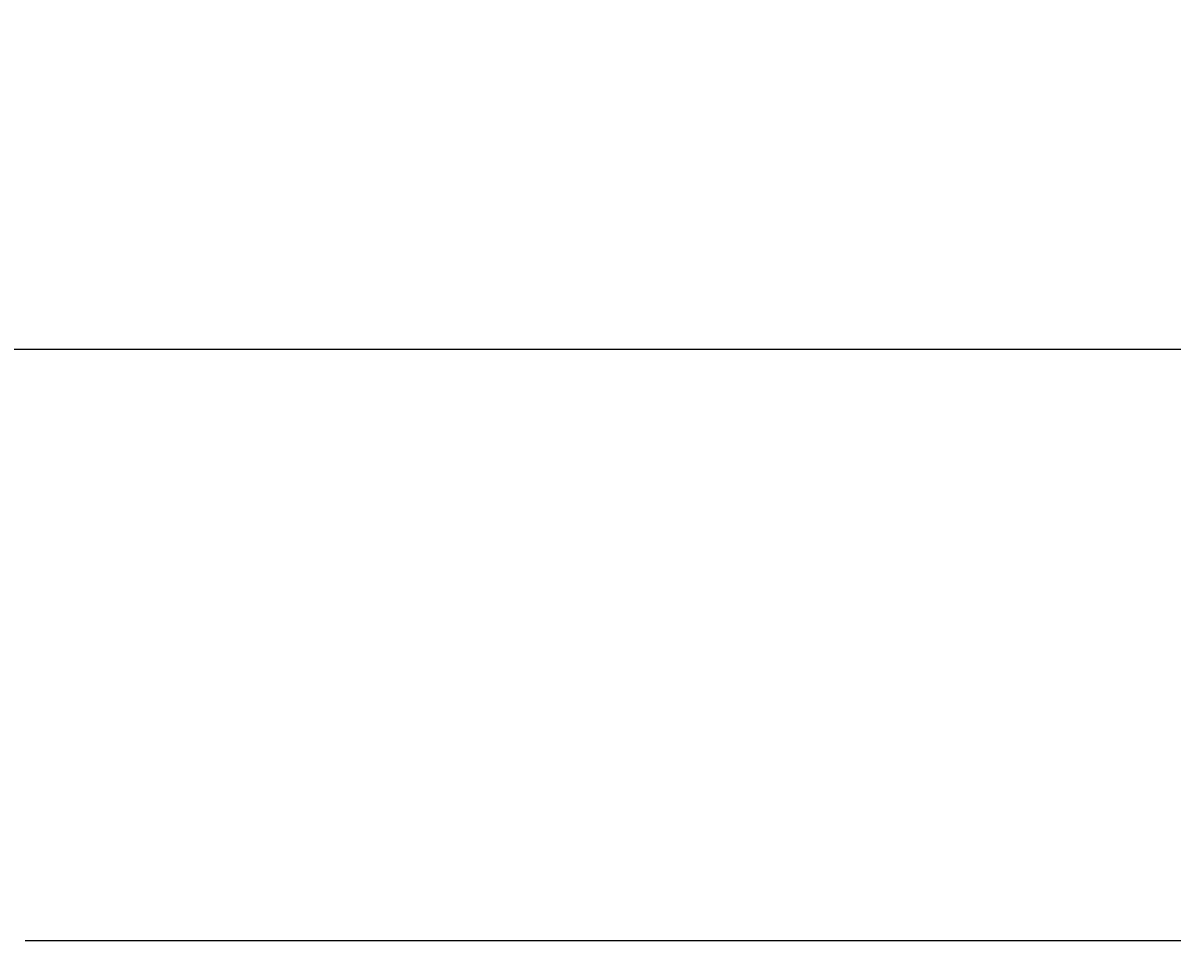
# Model space of a CAD drawing. Units: inches. Extents: x 1998 to 2588, y 1139 to 1977.
# Tile 11 of 134: x 2115 to 2147, y 1596 to 1622. Entities that reach past the tile are written whole.
import ezdxf

# ---------------------------------------------------------------- set-up
doc = ezdxf.new("R2010")
doc.units = ezdxf.units.IN
doc.layers.add('A-ANNO-DIMS', color=2, linetype='Continuous', lineweight=18)
doc.styles.get("Standard").update_dxf_attribs({"font": 'arial.ttf'})
doc.dimstyles.get("Standard").update_dxf_attribs({"dimtxt": 0.18, "dimasz": 0.18, "dimexe": 0.18, "dimexo": 0.0625, "dimgap": 0.09, "dimtad": 0, "dimtih": 1, "dimtoh": 1, "dimdec": 4, "dimzin": 0, "dimdsep": 46, "dimtxsty": 'Standard', "dimcen": 0.09, "dimadec": 0, "dimazin": 0, "dimtfac": 1, "dimtdec": 4, "dimtofl": 0, "dimtmove": 0, "dimatfit": 3, "dimfxl": 1, "dimtolj": 1, "dimtzin": 0, "dimarcsym": 0})

# ---------------------------------------------------------------- blocks, each defined once
blk = doc.blocks.new('*D30')
at = {"layer": 'A-ANNO-DIMS', "color": 0, "lineweight": -2, "transparency": 16777216}
for p, q in [((2407.91, 1636.732), (1997.843, 1636.732)), ((1998.023, 1636.552), (1998.023, 1615.913)), ((1998.023, 1594.912), (1998.023, 1615.552)), ((2407.91, 1594.732), (1997.843, 1594.732))]:
    blk.add_line(p, q, dxfattribs=at)
at = {"layer": 'A-ANNO-DIMS', "color": 0, "transparency": 16777216}
for points in [[(1997.993, 1636.552), (1998.053, 1636.552), (1998.023, 1636.732)], [(1997.993, 1594.912), (1998.053, 1594.912), (1998.023, 1594.732)]]:
    blk.add_solid(points, dxfattribs=at)
at = {"layer": 'Defpoints', "color": 0, "transparency": 16777216}
for p in [(1998.023, 1636.732), (2407.973, 1636.732), (2407.973, 1594.732)]:
    blk.add_point(p, dxfattribs=at)
at = {"layer": 'A-ANNO-DIMS', "color": 0, "transparency": 16777216, "insert": (1998.023, 1615.732), "char_height": 0.18, "attachment_point": 5}
blk.add_mtext('\\A1;42', dxfattribs=at)
blk = doc.blocks.new('*D35')
at = {"layer": 'A-ANNO-DIMS', "color": 0, "lineweight": -2, "transparency": 16777216}
for p, q in [((2148.392, 1612.732), (1997.843, 1612.732)), ((1998.023, 1612.552), (1998.023, 1600.913)), ((1998.023, 1588.912), (1998.023, 1600.552)), ((2148.392, 1588.732), (1997.843, 1588.732))]:
    blk.add_line(p, q, dxfattribs=at)
at = {"layer": 'A-ANNO-DIMS', "color": 0, "transparency": 16777216}
for points in [[(1997.993, 1612.552), (1998.053, 1612.552), (1998.023, 1612.732)], [(1997.993, 1588.912), (1998.053, 1588.912), (1998.023, 1588.732)]]:
    blk.add_solid(points, dxfattribs=at)
at = {"layer": 'Defpoints', "color": 0, "transparency": 16777216}
for p in [(1998.023, 1612.732), (2148.455, 1612.732), (2148.455, 1588.732)]:
    blk.add_point(p, dxfattribs=at)
at = {"layer": 'A-ANNO-DIMS', "color": 0, "transparency": 16777216, "insert": (1998.023, 1600.732), "char_height": 0.18, "attachment_point": 5}
blk.add_mtext('\\A1;24', dxfattribs=at)
blk = doc.blocks.new('*D38')
at = {"layer": 'A-ANNO-DIMS', "color": 0, "lineweight": -2, "transparency": 16777216}
for p, q in [((2197.387, 1663.247), (1997.843, 1663.247)), ((1998.023, 1663.067), (1998.023, 1638.171)), ((1998.023, 1612.912), (1998.023, 1637.808)), ((2197.387, 1612.732), (1997.843, 1612.732))]:
    blk.add_line(p, q, dxfattribs=at)
at = {"layer": 'A-ANNO-DIMS', "color": 0, "transparency": 16777216}
for points in [[(1997.993, 1663.067), (1998.053, 1663.067), (1998.023, 1663.247)], [(1997.993, 1612.912), (1998.053, 1612.912), (1998.023, 1612.732)]]:
    blk.add_solid(points, dxfattribs=at)
at = {"layer": 'Defpoints', "color": 0, "transparency": 16777216}
for p in [(1998.023, 1663.247), (2197.45, 1663.247), (2197.45, 1612.732)]:
    blk.add_point(p, dxfattribs=at)
at = {"layer": 'A-ANNO-DIMS', "color": 0, "transparency": 16777216, "insert": (1998.023, 1637.99), "char_height": 0.18, "attachment_point": 5}
blk.add_mtext('\\A1;50.51', dxfattribs=at)
blk = doc.blocks.new('*D39')
at = {"layer": 'A-ANNO-DIMS', "color": 0, "lineweight": -2, "transparency": 16777216}
for p, q in [((2115.035, 1628.742), (2588.309, 1628.742)), ((2588.129, 1628.562), (2588.129, 1612.685)), ((2588.129, 1596.444), (2588.129, 1612.321)), ((2115.035, 1596.264), (2588.309, 1596.264))]:
    blk.add_line(p, q, dxfattribs=at)
at = {"layer": 'A-ANNO-DIMS', "color": 0, "transparency": 16777216}
for points in [[(2588.099, 1628.562), (2588.159, 1628.562), (2588.129, 1628.742)], [(2588.099, 1596.444), (2588.159, 1596.444), (2588.129, 1596.264)]]:
    blk.add_solid(points, dxfattribs=at)
at = {"layer": 'Defpoints', "color": 0, "transparency": 16777216}
for p in [(2114.973, 1628.742), (2588.129, 1628.742), (2114.973, 1596.264)]:
    blk.add_point(p, dxfattribs=at)
at = {"layer": 'A-ANNO-DIMS', "color": 0, "transparency": 16777216, "insert": (2588.129, 1612.503), "char_height": 0.18, "attachment_point": 5}
blk.add_mtext('\\A1;32.48', dxfattribs=at)

msp = doc.modelspace()

# ---------------------------------------------------------------- dimensions: what is measured, and where the dimension line sits
at = {"layer": 'A-ANNO-DIMS'}
for base, p1, p2, override, picture, middle in [((1998.0229, 1663.2466), (2197.4499, 1612.7324), (2197.4499, 1663.2466), {"dimdec": 2, "dimlfac": 1, "dimrnd": 0, "dimzin": 0, "dimdsep": 46, "dimlunit": 2}, '*D38', (1998.0229, 1637.9895)), ((1998.0229, 1636.7324), (2407.9729, 1594.7324), (2407.9729, 1636.7324), {"dimdec": 0, "dimlfac": 1, "dimrnd": 0, "dimzin": 0, "dimdsep": 46, "dimlunit": 2}, '*D30', (1998.0229, 1615.7324)), ((2588.1286, 1628.7416), (2114.9729, 1596.2642), (2114.9729, 1628.7416), {"dimdec": 2, "dimlfac": 1, "dimrnd": 0, "dimzin": 0, "dimdsep": 46, "dimlunit": 2}, '*D39', (2588.1286, 1612.5029)), ((1998.0229, 1612.7324), (2148.4548, 1588.7324), (2148.4548, 1612.7324), {"dimdec": 0, "dimlfac": 1, "dimrnd": 0, "dimzin": 0, "dimdsep": 46, "dimlunit": 2}, '*D35', (1998.0229, 1600.7324))]:
    dim = msp.add_linear_dim(base=base, p1=p1, p2=p2, angle=90, dimstyle='Standard', override=override, dxfattribs=at)
    dim.commit()
    dim.dimension.update_dxf_attribs({"geometry": picture, "text_midpoint": middle})

doc.saveas('drawing.dxf')
